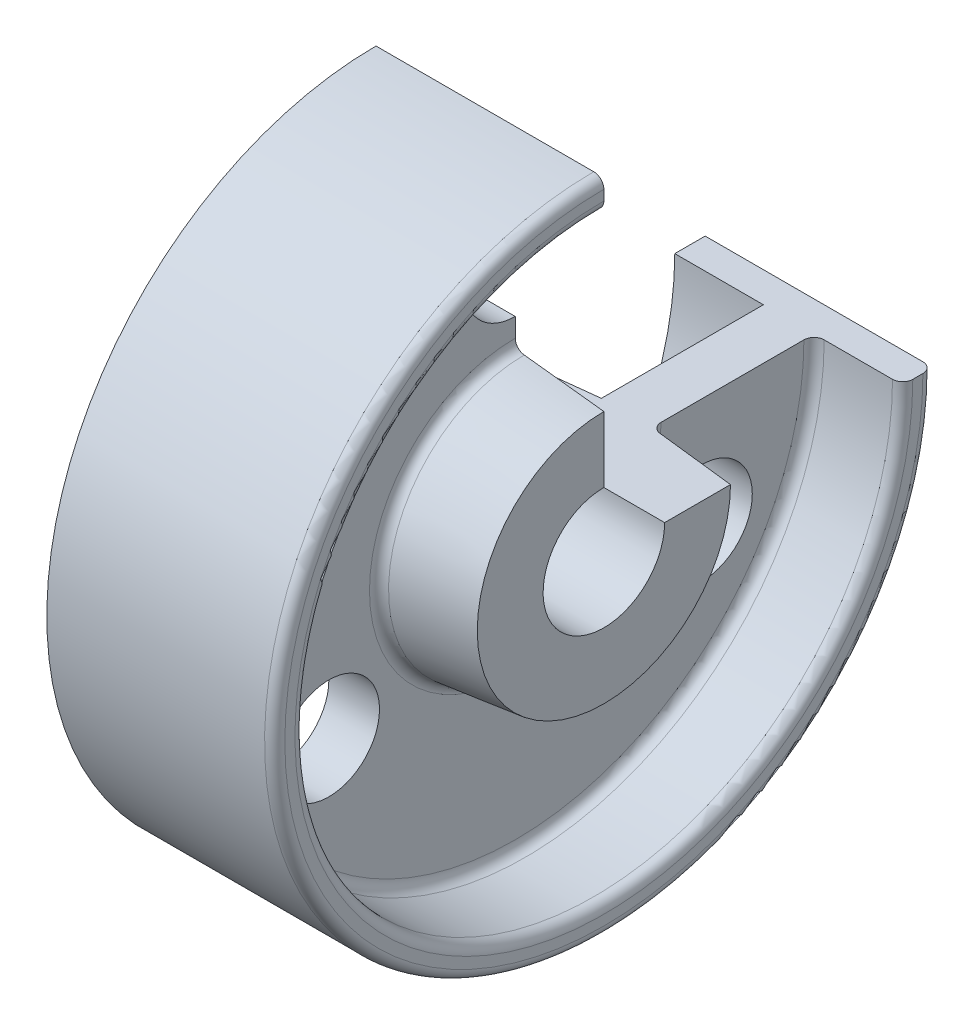
ISO-10303-21;
HEADER;
FILE_DESCRIPTION(('STEP AP214'),'2;1');
FILE_NAME('part.step','',(''),(''),'','','');
FILE_SCHEMA(('AUTOMOTIVE_DESIGN { 1 0 10303 214 1 1 1 1 }'));
ENDSEC;
DATA;
#1=APPLICATION_CONTEXT('core data for automotive mechanical design processes');
#2=APPLICATION_PROTOCOL_DEFINITION('international standard','automotive_design',2000,#1);
#3=PRODUCT_CONTEXT('',#1,'mechanical');
#4=PRODUCT('Part','Part','',(#3));
#5=PRODUCT_RELATED_PRODUCT_CATEGORY('part','',(#4));
#6=PRODUCT_DEFINITION_FORMATION('','',#4);
#7=PRODUCT_DEFINITION_CONTEXT('part definition',#1,'design');
#8=PRODUCT_DEFINITION('design','',#6,#7);
#9=PRODUCT_DEFINITION_SHAPE('','',#8);
#10=(LENGTH_UNIT() NAMED_UNIT(*) SI_UNIT(.MILLI.,.METRE.));
#11=(NAMED_UNIT(*) PLANE_ANGLE_UNIT() SI_UNIT($,.RADIAN.));
#12=(NAMED_UNIT(*) SI_UNIT($,.STERADIAN.) SOLID_ANGLE_UNIT());
#13=UNCERTAINTY_MEASURE_WITH_UNIT(LENGTH_MEASURE(1.E-05),#10,'distance_accuracy_value','');
#14=(GEOMETRIC_REPRESENTATION_CONTEXT(3) GLOBAL_UNCERTAINTY_ASSIGNED_CONTEXT((#13)) GLOBAL_UNIT_ASSIGNED_CONTEXT((#10,
#11,#12)) REPRESENTATION_CONTEXT('',''));
#15=CARTESIAN_POINT('',(0.,0.,0.));
#16=DIRECTION('',(0.,0.,1.));
#17=DIRECTION('',(1.,0.,0.));
#18=AXIS2_PLACEMENT_3D('',#15,#16,#17);
#19=CARTESIAN_POINT('',(5.,0.,0.));
#20=DIRECTION('',(-1.,0.,0.));
#21=DIRECTION('',(0.,0.,1.));
#22=AXIS2_PLACEMENT_3D('',#19,#20,#21);
#23=PLANE('',#22);
#24=CARTESIAN_POINT('',(5.,0.,0.));
#25=DIRECTION('',(-1.,0.,0.));
#26=DIRECTION('',(0.,0.,1.));
#27=AXIS2_PLACEMENT_3D('',#24,#25,#26);
#28=CIRCLE('',#27,57.);
#29=CARTESIAN_POINT('',(5.,57.,0.));
#30=VERTEX_POINT('',#29);
#31=CARTESIAN_POINT('',(5.,0.,-57.));
#32=VERTEX_POINT('',#31);
#33=EDGE_CURVE('E319',#30,#32,#28,.F.);
#34=ORIENTED_EDGE('',*,*,#33,.T.);
#35=DIRECTION('',(0.,0.,1.));
#36=VECTOR('',#35,1.);
#37=CARTESIAN_POINT('',(5.,0.,0.));
#38=LINE('',#37,#36);
#39=CARTESIAN_POINT('',(5.,0.,-28.7844474232924));
#40=VERTEX_POINT('',#39);
#41=EDGE_CURVE('E255',#32,#40,#38,.T.);
#42=ORIENTED_EDGE('',*,*,#41,.T.);
#43=CARTESIAN_POINT('',(5.,0.,0.));
#44=DIRECTION('',(-1.,0.,0.));
#45=DIRECTION('',(0.,0.,1.));
#46=AXIS2_PLACEMENT_3D('',#43,#44,#45);
#47=CIRCLE('',#46,28.7844474232924);
#48=CARTESIAN_POINT('',(5.,28.7844474232924,0.));
#49=VERTEX_POINT('',#48);
#50=EDGE_CURVE('E314',#40,#49,#47,.T.);
#51=ORIENTED_EDGE('',*,*,#50,.T.);
#52=DIRECTION('',(0.,1.,0.));
#53=VECTOR('',#52,1.);
#54=CARTESIAN_POINT('',(5.,0.,0.));
#55=LINE('',#54,#53);
#56=CARTESIAN_POINT('',(5.,32.5,0.));
#57=VERTEX_POINT('',#56);
#58=EDGE_CURVE('E57',#49,#57,#55,.T.);
#59=ORIENTED_EDGE('',*,*,#58,.T.);
#60=CARTESIAN_POINT('',(5.,42.5,0.));
#61=DIRECTION('',(1.,0.,0.));
#62=DIRECTION('',(0.,0.,-1.));
#63=AXIS2_PLACEMENT_3D('',#60,#61,#62);
#64=CIRCLE('',#63,10.);
#65=CARTESIAN_POINT('',(5.,52.5,0.));
#66=VERTEX_POINT('',#65);
#67=EDGE_CURVE('E271',#66,#57,#64,.T.);
#68=ORIENTED_EDGE('',*,*,#67,.F.);
#69=EDGE_CURVE('E221',#66,#30,#55,.T.);
#70=ORIENTED_EDGE('',*,*,#69,.T.);
#71=EDGE_LOOP('',(#34,#42,#51,#59,#68,#70));
#72=FACE_BOUND('',#71,.T.);
#73=CARTESIAN_POINT('',(5.,-21.250000000001,36.806079660838));
#74=DIRECTION('',(1.,0.,0.));
#75=DIRECTION('',(0.,0.,-1.));
#76=AXIS2_PLACEMENT_3D('',#73,#74,#75);
#77=CIRCLE('',#76,10.0000000000015);
#78=CARTESIAN_POINT('',(5.,-21.250000000001,26.8060796608365));
#79=VERTEX_POINT('',#78);
#80=EDGE_CURVE('E280',#79,#79,#77,.T.);
#81=ORIENTED_EDGE('',*,*,#80,.F.);
#82=EDGE_LOOP('',(#81));
#83=FACE_BOUND('',#82,.T.);
#84=CARTESIAN_POINT('',(5.,-21.25,-36.8060796608398));
#85=DIRECTION('',(1.,0.,0.));
#86=DIRECTION('',(0.,0.,-1.));
#87=AXIS2_PLACEMENT_3D('',#84,#85,#86);
#88=CIRCLE('',#87,10.0000000000005);
#89=CARTESIAN_POINT('',(5.,-21.25,-46.8060796608403));
#90=VERTEX_POINT('',#89);
#91=EDGE_CURVE('E275',#90,#90,#88,.T.);
#92=ORIENTED_EDGE('',*,*,#91,.F.);
#93=EDGE_LOOP('',(#92));
#94=FACE_BOUND('',#93,.T.);
#95=ADVANCED_FACE('F41',(#72,#83,#94),#23,.F.);
#96=CARTESIAN_POINT('',(-22.5,0.,0.));
#97=DIRECTION('',(-1.,0.,0.));
#98=DIRECTION('',(0.,0.,1.));
#99=AXIS2_PLACEMENT_3D('',#96,#97,#98);
#100=PLANE('',#99);
#101=DIRECTION('',(0.,0.,-1.));
#102=VECTOR('',#101,1.);
#103=CARTESIAN_POINT('',(-22.5,0.,0.));
#104=LINE('',#103,#102);
#105=CARTESIAN_POINT('',(-22.5,0.,-12.));
#106=VERTEX_POINT('',#105);
#107=CARTESIAN_POINT('',(-22.5,0.,-25.));
#108=VERTEX_POINT('',#107);
#109=EDGE_CURVE('E206',#106,#108,#104,.T.);
#110=ORIENTED_EDGE('',*,*,#109,.T.);
#111=CARTESIAN_POINT('',(-22.5,0.,0.));
#112=DIRECTION('',(-1.,0.,0.));
#113=DIRECTION('',(0.,0.,1.));
#114=AXIS2_PLACEMENT_3D('',#111,#112,#113);
#115=CIRCLE('',#114,25.);
#116=CARTESIAN_POINT('',(-22.5,25.,0.));
#117=VERTEX_POINT('',#116);
#118=EDGE_CURVE('E281',#108,#117,#115,.T.);
#119=ORIENTED_EDGE('',*,*,#118,.T.);
#120=DIRECTION('',(0.,-1.,0.));
#121=VECTOR('',#120,1.);
#122=CARTESIAN_POINT('',(-22.5,77.9926066109058,0.));
#123=LINE('',#122,#121);
#124=CARTESIAN_POINT('',(-22.5,12.,0.));
#125=VERTEX_POINT('',#124);
#126=EDGE_CURVE('E219',#117,#125,#123,.T.);
#127=ORIENTED_EDGE('',*,*,#126,.T.);
#128=CARTESIAN_POINT('',(-22.5,0.,0.));
#129=DIRECTION('',(-1.,0.,0.));
#130=DIRECTION('',(0.,0.,1.));
#131=AXIS2_PLACEMENT_3D('',#128,#129,#130);
#132=CIRCLE('',#131,12.);
#133=EDGE_CURVE('E302',#106,#125,#132,.T.);
#134=ORIENTED_EDGE('',*,*,#133,.F.);
#135=EDGE_LOOP('',(#110,#119,#127,#134));
#136=FACE_BOUND('',#135,.T.);
#137=ADVANCED_FACE('F366',(#136),#100,.T.);
#138=CARTESIAN_POINT('',(-53.0847305724635,0.,0.));
#139=DIRECTION('',(-1.,0.,0.));
#140=DIRECTION('',(0.,0.,1.));
#141=AXIS2_PLACEMENT_3D('',#138,#139,#140);
#142=CYLINDRICAL_SURFACE('',#141,12.);
#143=DIRECTION('',(-1.,0.,0.));
#144=VECTOR('',#143,1.);
#145=CARTESIAN_POINT('',(-53.0847305724635,0.,-12.));
#146=LINE('',#145,#144);
#147=CARTESIAN_POINT('',(22.5,0.,-12.));
#148=VERTEX_POINT('',#147);
#149=EDGE_CURVE('E266',#106,#148,#146,.F.);
#150=ORIENTED_EDGE('',*,*,#149,.F.);
#151=ORIENTED_EDGE('',*,*,#133,.T.);
#152=DIRECTION('',(-1.,0.,0.));
#153=VECTOR('',#152,1.);
#154=CARTESIAN_POINT('',(-53.0847305724635,12.,0.));
#155=LINE('',#154,#153);
#156=CARTESIAN_POINT('',(22.5,12.,0.));
#157=VERTEX_POINT('',#156);
#158=EDGE_CURVE('E246',#157,#125,#155,.T.);
#159=ORIENTED_EDGE('',*,*,#158,.F.);
#160=CARTESIAN_POINT('',(22.5,0.,0.));
#161=DIRECTION('',(-1.,0.,0.));
#162=DIRECTION('',(0.,0.,1.));
#163=AXIS2_PLACEMENT_3D('',#160,#161,#162);
#164=CIRCLE('',#163,12.);
#165=EDGE_CURVE('E301',#148,#157,#164,.T.);
#166=ORIENTED_EDGE('',*,*,#165,.F.);
#167=EDGE_LOOP('',(#150,#151,#159,#166));
#168=FACE_BOUND('',#167,.T.);
#169=ADVANCED_FACE('F367',(#168),#142,.F.);
#170=CARTESIAN_POINT('',(22.5,0.,0.));
#171=DIRECTION('',(-1.,0.,0.));
#172=DIRECTION('',(0.,0.,1.));
#173=AXIS2_PLACEMENT_3D('',#170,#171,#172);
#174=PLANE('',#173);
#175=CARTESIAN_POINT('',(22.5,0.,0.));
#176=DIRECTION('',(-1.,0.,0.));
#177=DIRECTION('',(0.,0.,1.));
#178=AXIS2_PLACEMENT_3D('',#175,#176,#177);
#179=CIRCLE('',#178,25.);
#180=CARTESIAN_POINT('',(22.5,0.,-25.));
#181=VERTEX_POINT('',#180);
#182=CARTESIAN_POINT('',(22.5,25.,0.));
#183=VERTEX_POINT('',#182);
#184=EDGE_CURVE('E296',#181,#183,#179,.T.);
#185=ORIENTED_EDGE('',*,*,#184,.F.);
#186=DIRECTION('',(0.,0.,-1.));
#187=VECTOR('',#186,1.);
#188=CARTESIAN_POINT('',(22.5,0.,0.));
#189=LINE('',#188,#187);
#190=EDGE_CURVE('E211',#148,#181,#189,.T.);
#191=ORIENTED_EDGE('',*,*,#190,.F.);
#192=ORIENTED_EDGE('',*,*,#165,.T.);
#193=DIRECTION('',(0.,-1.,0.));
#194=VECTOR('',#193,1.);
#195=CARTESIAN_POINT('',(22.5,77.9926066109058,0.));
#196=LINE('',#195,#194);
#197=EDGE_CURVE('E185',#183,#157,#196,.T.);
#198=ORIENTED_EDGE('',*,*,#197,.F.);
#199=EDGE_LOOP('',(#185,#191,#192,#198));
#200=FACE_BOUND('',#199,.T.);
#201=ADVANCED_FACE('F373',(#200),#174,.F.);
#202=CARTESIAN_POINT('',(22.5,0.,0.));
#203=DIRECTION('',(-1.,0.,0.));
#204=DIRECTION('',(0.,0.,1.));
#205=AXIS2_PLACEMENT_3D('',#202,#203,#204);
#206=CONICAL_SURFACE('',#205,25.,0.113792007143708);
#207=CARTESIAN_POINT('',(6.77290681767853,0.,0.));
#208=DIRECTION('',(-1.,0.,0.));
#209=DIRECTION('',(0.,0.,1.));
#210=AXIS2_PLACEMENT_3D('',#207,#208,#209);
#211=CIRCLE('',#210,26.7973820779796);
#212=CARTESIAN_POINT('',(6.77290681767853,26.7973820779796,0.));
#213=VERTEX_POINT('',#212);
#214=CARTESIAN_POINT('',(6.77290681767853,0.,-26.7973820779796));
#215=VERTEX_POINT('',#214);
#216=EDGE_CURVE('E192',#213,#215,#211,.F.);
#217=ORIENTED_EDGE('',*,*,#216,.T.);
#218=DIRECTION('',(0.993532672656404,0.,0.113546591160732));
#219=VECTOR('',#218,1.);
#220=CARTESIAN_POINT('',(241.25,0.,0.));
#221=LINE('',#220,#219);
#222=EDGE_CURVE('E259',#215,#181,#221,.T.);
#223=ORIENTED_EDGE('',*,*,#222,.T.);
#224=ORIENTED_EDGE('',*,*,#184,.T.);
#225=DIRECTION('',(-0.993532672656404,0.113546591160732,0.));
#226=VECTOR('',#225,1.);
#227=CARTESIAN_POINT('',(241.25,0.,0.));
#228=LINE('',#227,#226);
#229=EDGE_CURVE('E238',#183,#213,#228,.T.);
#230=ORIENTED_EDGE('',*,*,#229,.T.);
#231=EDGE_LOOP('',(#217,#223,#224,#230));
#232=FACE_BOUND('',#231,.T.);
#233=ADVANCED_FACE('F324',(#232),#206,.T.);
#234=CARTESIAN_POINT('',(-53.0847305724635,0.,0.));
#235=DIRECTION('',(-1.,0.,0.));
#236=DIRECTION('',(0.,0.,1.));
#237=AXIS2_PLACEMENT_3D('',#234,#235,#236);
#238=CYLINDRICAL_SURFACE('',#237,59.);
#239=CARTESIAN_POINT('',(20.5,0.,0.));
#240=DIRECTION('',(-1.,0.,0.));
#241=DIRECTION('',(0.,0.,1.));
#242=AXIS2_PLACEMENT_3D('',#239,#240,#241);
#243=CIRCLE('',#242,59.);
#244=CARTESIAN_POINT('',(20.5,59.,0.));
#245=VERTEX_POINT('',#244);
#246=CARTESIAN_POINT('',(20.5,0.,-59.));
#247=VERTEX_POINT('',#246);
#248=EDGE_CURVE('E186',#245,#247,#243,.F.);
#249=ORIENTED_EDGE('',*,*,#248,.T.);
#250=DIRECTION('',(-1.,0.,0.));
#251=VECTOR('',#250,1.);
#252=CARTESIAN_POINT('',(-53.0847305724635,0.,-59.));
#253=LINE('',#252,#251);
#254=CARTESIAN_POINT('',(7.,0.,-59.));
#255=VERTEX_POINT('',#254);
#256=EDGE_CURVE('E214',#247,#255,#253,.T.);
#257=ORIENTED_EDGE('',*,*,#256,.T.);
#258=CARTESIAN_POINT('',(7.,0.,0.));
#259=DIRECTION('',(-1.,0.,0.));
#260=DIRECTION('',(0.,0.,1.));
#261=AXIS2_PLACEMENT_3D('',#258,#259,#260);
#262=CIRCLE('',#261,59.);
#263=CARTESIAN_POINT('',(7.,59.,0.));
#264=VERTEX_POINT('',#263);
#265=EDGE_CURVE('E207',#255,#264,#262,.T.);
#266=ORIENTED_EDGE('',*,*,#265,.T.);
#267=DIRECTION('',(-1.,0.,0.));
#268=VECTOR('',#267,1.);
#269=CARTESIAN_POINT('',(-53.0847305724635,59.,0.));
#270=LINE('',#269,#268);
#271=EDGE_CURVE('E196',#264,#245,#270,.F.);
#272=ORIENTED_EDGE('',*,*,#271,.T.);
#273=EDGE_LOOP('',(#249,#257,#266,#272));
#274=FACE_BOUND('',#273,.T.);
#275=ADVANCED_FACE('F202',(#274),#238,.F.);
#276=CARTESIAN_POINT('',(22.5,0.,0.));
#277=DIRECTION('',(-1.,0.,0.));
#278=DIRECTION('',(0.,0.,1.));
#279=AXIS2_PLACEMENT_3D('',#276,#277,#278);
#280=PLANE('',#279);
#281=CARTESIAN_POINT('',(22.5,0.,0.));
#282=DIRECTION('',(-1.,0.,0.));
#283=DIRECTION('',(0.,0.,1.));
#284=AXIS2_PLACEMENT_3D('',#281,#282,#283);
#285=CIRCLE('',#284,63.);
#286=CARTESIAN_POINT('',(22.5,63.,0.));
#287=VERTEX_POINT('',#286);
#288=CARTESIAN_POINT('',(22.5,0.,-63.));
#289=VERTEX_POINT('',#288);
#290=EDGE_CURVE('E178',#287,#289,#285,.F.);
#291=ORIENTED_EDGE('',*,*,#290,.T.);
#292=CARTESIAN_POINT('',(22.5,0.,-61.));
#293=VERTEX_POINT('',#292);
#294=EDGE_CURVE('E181',#293,#289,#189,.T.);
#295=ORIENTED_EDGE('',*,*,#294,.F.);
#296=CARTESIAN_POINT('',(22.5,0.,0.));
#297=DIRECTION('',(-1.,0.,0.));
#298=DIRECTION('',(0.,0.,1.));
#299=AXIS2_PLACEMENT_3D('',#296,#297,#298);
#300=CIRCLE('',#299,61.);
#301=CARTESIAN_POINT('',(22.5,61.,0.));
#302=VERTEX_POINT('',#301);
#303=EDGE_CURVE('E179',#293,#302,#300,.T.);
#304=ORIENTED_EDGE('',*,*,#303,.T.);
#305=EDGE_CURVE('E61',#287,#302,#196,.T.);
#306=ORIENTED_EDGE('',*,*,#305,.F.);
#307=EDGE_LOOP('',(#291,#295,#304,#306));
#308=FACE_BOUND('',#307,.T.);
#309=ADVANCED_FACE('F176',(#308),#280,.F.);
#310=CARTESIAN_POINT('',(-53.0847305724635,0.,0.));
#311=DIRECTION('',(-1.,0.,0.));
#312=DIRECTION('',(0.,0.,1.));
#313=AXIS2_PLACEMENT_3D('',#310,#311,#312);
#314=CYLINDRICAL_SURFACE('',#313,65.);
#315=DIRECTION('',(-1.,0.,0.));
#316=VECTOR('',#315,1.);
#317=CARTESIAN_POINT('',(-53.0847305724635,0.,-65.));
#318=LINE('',#317,#316);
#319=CARTESIAN_POINT('',(20.5,0.,-65.));
#320=VERTEX_POINT('',#319);
#321=CARTESIAN_POINT('',(-22.5,0.,-65.));
#322=VERTEX_POINT('',#321);
#323=EDGE_CURVE('E261',#320,#322,#318,.T.);
#324=ORIENTED_EDGE('',*,*,#323,.F.);
#325=CARTESIAN_POINT('',(20.5,0.,0.));
#326=DIRECTION('',(-1.,0.,0.));
#327=DIRECTION('',(0.,0.,1.));
#328=AXIS2_PLACEMENT_3D('',#325,#326,#327);
#329=CIRCLE('',#328,65.);
#330=CARTESIAN_POINT('',(20.5,65.,0.));
#331=VERTEX_POINT('',#330);
#332=EDGE_CURVE('E190',#320,#331,#329,.T.);
#333=ORIENTED_EDGE('',*,*,#332,.T.);
#334=DIRECTION('',(-1.,0.,0.));
#335=VECTOR('',#334,1.);
#336=CARTESIAN_POINT('',(-53.0847305724635,65.,0.));
#337=LINE('',#336,#335);
#338=CARTESIAN_POINT('',(-22.5,65.,0.));
#339=VERTEX_POINT('',#338);
#340=EDGE_CURVE('E168',#339,#331,#337,.F.);
#341=ORIENTED_EDGE('',*,*,#340,.F.);
#342=CARTESIAN_POINT('',(-22.5,0.,0.));
#343=DIRECTION('',(-1.,0.,0.));
#344=DIRECTION('',(0.,0.,1.));
#345=AXIS2_PLACEMENT_3D('',#342,#343,#344);
#346=CIRCLE('',#345,65.);
#347=EDGE_CURVE('E294',#322,#339,#346,.T.);
#348=ORIENTED_EDGE('',*,*,#347,.F.);
#349=EDGE_LOOP('',(#324,#333,#341,#348));
#350=FACE_BOUND('',#349,.T.);
#351=ADVANCED_FACE('F358',(#350),#314,.T.);
#352=CARTESIAN_POINT('',(-22.5,0.,0.));
#353=DIRECTION('',(-1.,0.,0.));
#354=DIRECTION('',(0.,0.,1.));
#355=AXIS2_PLACEMENT_3D('',#352,#353,#354);
#356=PLANE('',#355);
#357=CARTESIAN_POINT('',(-22.5,0.,-59.));
#358=VERTEX_POINT('',#357);
#359=EDGE_CURVE('E223',#358,#322,#104,.T.);
#360=ORIENTED_EDGE('',*,*,#359,.T.);
#361=ORIENTED_EDGE('',*,*,#347,.T.);
#362=CARTESIAN_POINT('',(-22.5,59.,0.));
#363=VERTEX_POINT('',#362);
#364=EDGE_CURVE('E217',#339,#363,#123,.T.);
#365=ORIENTED_EDGE('',*,*,#364,.T.);
#366=CARTESIAN_POINT('',(-22.5,0.,0.));
#367=DIRECTION('',(-1.,0.,0.));
#368=DIRECTION('',(0.,0.,1.));
#369=AXIS2_PLACEMENT_3D('',#366,#367,#368);
#370=CIRCLE('',#369,59.);
#371=EDGE_CURVE('E292',#358,#363,#370,.T.);
#372=ORIENTED_EDGE('',*,*,#371,.F.);
#373=EDGE_LOOP('',(#360,#361,#365,#372));
#374=FACE_BOUND('',#373,.T.);
#375=ADVANCED_FACE('F354',(#374),#356,.T.);
#376=CARTESIAN_POINT('',(-53.0847305724635,0.,0.));
#377=DIRECTION('',(-1.,0.,0.));
#378=DIRECTION('',(0.,0.,1.));
#379=AXIS2_PLACEMENT_3D('',#376,#377,#378);
#380=CYLINDRICAL_SURFACE('',#379,59.);
#381=DIRECTION('',(-1.,0.,0.));
#382=VECTOR('',#381,1.);
#383=CARTESIAN_POINT('',(-53.0847305724635,0.,-59.));
#384=LINE('',#383,#382);
#385=CARTESIAN_POINT('',(-5.,0.,-59.));
#386=VERTEX_POINT('',#385);
#387=EDGE_CURVE('E267',#358,#386,#384,.F.);
#388=ORIENTED_EDGE('',*,*,#387,.F.);
#389=ORIENTED_EDGE('',*,*,#371,.T.);
#390=DIRECTION('',(-1.,0.,0.));
#391=VECTOR('',#390,1.);
#392=CARTESIAN_POINT('',(-53.0847305724635,59.,0.));
#393=LINE('',#392,#391);
#394=CARTESIAN_POINT('',(-5.,59.,0.));
#395=VERTEX_POINT('',#394);
#396=EDGE_CURVE('E171',#395,#363,#393,.T.);
#397=ORIENTED_EDGE('',*,*,#396,.F.);
#398=CARTESIAN_POINT('',(-5.,0.,0.));
#399=DIRECTION('',(-1.,0.,0.));
#400=DIRECTION('',(0.,0.,1.));
#401=AXIS2_PLACEMENT_3D('',#398,#399,#400);
#402=CIRCLE('',#401,59.);
#403=EDGE_CURVE('E290',#386,#395,#402,.T.);
#404=ORIENTED_EDGE('',*,*,#403,.F.);
#405=EDGE_LOOP('',(#388,#389,#397,#404));
#406=FACE_BOUND('',#405,.T.);
#407=ADVANCED_FACE('F348',(#406),#380,.F.);
#408=CARTESIAN_POINT('',(-5.,0.,0.));
#409=DIRECTION('',(-1.,0.,0.));
#410=DIRECTION('',(0.,0.,1.));
#411=AXIS2_PLACEMENT_3D('',#408,#409,#410);
#412=PLANE('',#411);
#413=DIRECTION('',(0.,0.,1.));
#414=VECTOR('',#413,1.);
#415=CARTESIAN_POINT('',(-5.,0.,0.));
#416=LINE('',#415,#414);
#417=CARTESIAN_POINT('',(-5.,0.,-27.));
#418=VERTEX_POINT('',#417);
#419=EDGE_CURVE('E268',#386,#418,#416,.T.);
#420=ORIENTED_EDGE('',*,*,#419,.F.);
#421=ORIENTED_EDGE('',*,*,#403,.T.);
#422=DIRECTION('',(0.,1.,0.));
#423=VECTOR('',#422,1.);
#424=CARTESIAN_POINT('',(-5.,0.,0.));
#425=LINE('',#424,#423);
#426=CARTESIAN_POINT('',(-5.,52.5,0.));
#427=VERTEX_POINT('',#426);
#428=EDGE_CURVE('E233',#427,#395,#425,.T.);
#429=ORIENTED_EDGE('',*,*,#428,.F.);
#430=CARTESIAN_POINT('',(-5.,42.5,0.));
#431=DIRECTION('',(-1.,0.,0.));
#432=DIRECTION('',(0.,0.,1.));
#433=AXIS2_PLACEMENT_3D('',#430,#431,#432);
#434=CIRCLE('',#433,10.);
#435=CARTESIAN_POINT('',(-5.,32.5,0.));
#436=VERTEX_POINT('',#435);
#437=EDGE_CURVE('E288',#436,#427,#434,.T.);
#438=ORIENTED_EDGE('',*,*,#437,.F.);
#439=CARTESIAN_POINT('',(-5.,27.,0.));
#440=VERTEX_POINT('',#439);
#441=EDGE_CURVE('E231',#440,#436,#425,.T.);
#442=ORIENTED_EDGE('',*,*,#441,.F.);
#443=CARTESIAN_POINT('',(-5.,0.,0.));
#444=DIRECTION('',(-1.,0.,0.));
#445=DIRECTION('',(0.,0.,1.));
#446=AXIS2_PLACEMENT_3D('',#443,#444,#445);
#447=CIRCLE('',#446,27.);
#448=EDGE_CURVE('E282',#418,#440,#447,.T.);
#449=ORIENTED_EDGE('',*,*,#448,.F.);
#450=EDGE_LOOP('',(#420,#421,#429,#438,#442,#449));
#451=FACE_BOUND('',#450,.T.);
#452=CARTESIAN_POINT('',(-5.,-21.250000000001,36.806079660838));
#453=DIRECTION('',(-1.,0.,0.));
#454=DIRECTION('',(0.,0.,1.));
#455=AXIS2_PLACEMENT_3D('',#452,#453,#454);
#456=CIRCLE('',#455,10.0000000000015);
#457=CARTESIAN_POINT('',(-5.,-21.250000000001,46.8060796608396));
#458=VERTEX_POINT('',#457);
#459=EDGE_CURVE('E307',#458,#458,#456,.T.);
#460=ORIENTED_EDGE('',*,*,#459,.F.);
#461=EDGE_LOOP('',(#460));
#462=FACE_BOUND('',#461,.T.);
#463=CARTESIAN_POINT('',(-5.,-21.25,-36.8060796608398));
#464=DIRECTION('',(-1.,0.,0.));
#465=DIRECTION('',(0.,0.,1.));
#466=AXIS2_PLACEMENT_3D('',#463,#464,#465);
#467=CIRCLE('',#466,10.0000000000005);
#468=CARTESIAN_POINT('',(-5.,-21.25,-26.8060796608393));
#469=VERTEX_POINT('',#468);
#470=EDGE_CURVE('E277',#469,#469,#467,.T.);
#471=ORIENTED_EDGE('',*,*,#470,.F.);
#472=EDGE_LOOP('',(#471));
#473=FACE_BOUND('',#472,.T.);
#474=ADVANCED_FACE('F342',(#451,#462,#473),#412,.T.);
#475=CARTESIAN_POINT('',(-22.5,0.,0.));
#476=DIRECTION('',(1.,0.,0.));
#477=DIRECTION('',(0.,0.,-1.));
#478=AXIS2_PLACEMENT_3D('',#475,#476,#477);
#479=CONICAL_SURFACE('',#478,25.,0.113792007143708);
#480=DIRECTION('',(0.993532672656404,0.,-0.113546591160732));
#481=VECTOR('',#480,1.);
#482=CARTESIAN_POINT('',(-241.250000000001,0.,0.));
#483=LINE('',#482,#481);
#484=EDGE_CURVE('E263',#418,#108,#483,.F.);
#485=ORIENTED_EDGE('',*,*,#484,.F.);
#486=ORIENTED_EDGE('',*,*,#448,.T.);
#487=DIRECTION('',(-0.993532672656404,-0.113546591160732,0.));
#488=VECTOR('',#487,1.);
#489=CARTESIAN_POINT('',(-241.250000000001,0.,0.));
#490=LINE('',#489,#488);
#491=EDGE_CURVE('E242',#117,#440,#490,.F.);
#492=ORIENTED_EDGE('',*,*,#491,.F.);
#493=ORIENTED_EDGE('',*,*,#118,.F.);
#494=EDGE_LOOP('',(#485,#486,#492,#493));
#495=FACE_BOUND('',#494,.T.);
#496=ADVANCED_FACE('F359',(#495),#479,.T.);
#497=CARTESIAN_POINT('',(-22.5,-21.25,-36.8060796608398));
#498=DIRECTION('',(1.,0.,0.));
#499=DIRECTION('',(0.,0.,-1.));
#500=AXIS2_PLACEMENT_3D('',#497,#498,#499);
#501=CYLINDRICAL_SURFACE('',#500,10.0000000000005);
#502=ORIENTED_EDGE('',*,*,#470,.T.);
#503=EDGE_LOOP('',(#502));
#504=FACE_BOUND('',#503,.T.);
#505=ORIENTED_EDGE('',*,*,#91,.T.);
#506=EDGE_LOOP('',(#505));
#507=FACE_BOUND('',#506,.T.);
#508=ADVANCED_FACE('F451',(#504,#507),#501,.F.);
#509=CARTESIAN_POINT('',(-22.5,-21.250000000001,36.806079660838));
#510=DIRECTION('',(1.,0.,0.));
#511=DIRECTION('',(0.,0.,-1.));
#512=AXIS2_PLACEMENT_3D('',#509,#510,#511);
#513=CYLINDRICAL_SURFACE('',#512,10.0000000000015);
#514=ORIENTED_EDGE('',*,*,#459,.T.);
#515=EDGE_LOOP('',(#514));
#516=FACE_BOUND('',#515,.T.);
#517=ORIENTED_EDGE('',*,*,#80,.T.);
#518=EDGE_LOOP('',(#517));
#519=FACE_BOUND('',#518,.T.);
#520=ADVANCED_FACE('F449',(#516,#519),#513,.F.);
#521=CARTESIAN_POINT('',(-22.5,42.5,0.));
#522=DIRECTION('',(1.,0.,0.));
#523=DIRECTION('',(0.,0.,-1.));
#524=AXIS2_PLACEMENT_3D('',#521,#522,#523);
#525=CYLINDRICAL_SURFACE('',#524,10.);
#526=ORIENTED_EDGE('',*,*,#67,.T.);
#527=DIRECTION('',(1.,0.,0.));
#528=VECTOR('',#527,1.);
#529=CARTESIAN_POINT('',(-22.5,32.5,0.));
#530=LINE('',#529,#528);
#531=EDGE_CURVE('E241',#57,#436,#530,.F.);
#532=ORIENTED_EDGE('',*,*,#531,.T.);
#533=ORIENTED_EDGE('',*,*,#437,.T.);
#534=DIRECTION('',(1.,0.,0.));
#535=VECTOR('',#534,1.);
#536=CARTESIAN_POINT('',(-22.5,52.5,0.));
#537=LINE('',#536,#535);
#538=EDGE_CURVE('E226',#427,#66,#537,.T.);
#539=ORIENTED_EDGE('',*,*,#538,.T.);
#540=EDGE_LOOP('',(#526,#532,#533,#539));
#541=FACE_BOUND('',#540,.T.);
#542=ADVANCED_FACE('F337',(#541),#525,.F.);
#543=CARTESIAN_POINT('',(7.,0.,0.));
#544=DIRECTION('',(-1.,0.,0.));
#545=DIRECTION('',(0.,0.,1.));
#546=AXIS2_PLACEMENT_3D('',#543,#544,#545);
#547=TOROIDAL_SURFACE('',#546,57.,2.);
#548=ORIENTED_EDGE('',*,*,#265,.F.);
#549=CARTESIAN_POINT('',(7.,0.,-57.));
#550=DIRECTION('',(0.,-1.,0.));
#551=DIRECTION('',(0.,0.,-1.));
#552=AXIS2_PLACEMENT_3D('',#549,#550,#551);
#553=CIRCLE('',#552,2.);
#554=EDGE_CURVE('E248',#255,#32,#553,.F.);
#555=ORIENTED_EDGE('',*,*,#554,.T.);
#556=ORIENTED_EDGE('',*,*,#33,.F.);
#557=CARTESIAN_POINT('',(7.,57.,0.));
#558=DIRECTION('',(0.,0.,1.));
#559=DIRECTION('',(1.,0.,0.));
#560=AXIS2_PLACEMENT_3D('',#557,#558,#559);
#561=CIRCLE('',#560,2.);
#562=EDGE_CURVE('E210',#30,#264,#561,.F.);
#563=ORIENTED_EDGE('',*,*,#562,.T.);
#564=EDGE_LOOP('',(#548,#555,#556,#563));
#565=FACE_BOUND('',#564,.T.);
#566=ADVANCED_FACE('F332',(#565),#547,.F.);
#567=CARTESIAN_POINT('',(7.,0.,0.));
#568=DIRECTION('',(-1.,0.,0.));
#569=DIRECTION('',(0.,0.,1.));
#570=AXIS2_PLACEMENT_3D('',#567,#568,#569);
#571=TOROIDAL_SURFACE('',#570,28.7844474232924,2.);
#572=ORIENTED_EDGE('',*,*,#50,.F.);
#573=CARTESIAN_POINT('',(7.,0.,-28.7844474232924));
#574=DIRECTION('',(0.,-1.,0.));
#575=DIRECTION('',(0.,0.,-1.));
#576=AXIS2_PLACEMENT_3D('',#573,#574,#575);
#577=CIRCLE('',#576,2.);
#578=EDGE_CURVE('E253',#40,#215,#577,.F.);
#579=ORIENTED_EDGE('',*,*,#578,.T.);
#580=ORIENTED_EDGE('',*,*,#216,.F.);
#581=CARTESIAN_POINT('',(7.,28.7844474232924,0.));
#582=DIRECTION('',(0.,0.,1.));
#583=DIRECTION('',(1.,0.,0.));
#584=AXIS2_PLACEMENT_3D('',#581,#582,#583);
#585=CIRCLE('',#584,2.);
#586=EDGE_CURVE('E236',#213,#49,#585,.F.);
#587=ORIENTED_EDGE('',*,*,#586,.T.);
#588=EDGE_LOOP('',(#572,#579,#580,#587));
#589=FACE_BOUND('',#588,.T.);
#590=ADVANCED_FACE('F326',(#589),#571,.F.);
#591=CARTESIAN_POINT('',(20.5,0.,0.));
#592=DIRECTION('',(-1.,0.,0.));
#593=DIRECTION('',(0.,0.,1.));
#594=AXIS2_PLACEMENT_3D('',#591,#592,#593);
#595=TOROIDAL_SURFACE('',#594,63.,2.);
#596=CARTESIAN_POINT('',(20.5,0.,-63.));
#597=DIRECTION('',(0.,-1.,0.));
#598=DIRECTION('',(0.,0.,-1.));
#599=AXIS2_PLACEMENT_3D('',#596,#597,#598);
#600=CIRCLE('',#599,2.);
#601=EDGE_CURVE('E187',#289,#320,#600,.F.);
#602=ORIENTED_EDGE('',*,*,#601,.F.);
#603=ORIENTED_EDGE('',*,*,#290,.F.);
#604=CARTESIAN_POINT('',(20.5,63.,0.));
#605=DIRECTION('',(0.,0.,1.));
#606=DIRECTION('',(1.,0.,0.));
#607=AXIS2_PLACEMENT_3D('',#604,#605,#606);
#608=CIRCLE('',#607,2.);
#609=EDGE_CURVE('E161',#331,#287,#608,.F.);
#610=ORIENTED_EDGE('',*,*,#609,.F.);
#611=ORIENTED_EDGE('',*,*,#332,.F.);
#612=EDGE_LOOP('',(#602,#603,#610,#611));
#613=FACE_BOUND('',#612,.T.);
#614=ADVANCED_FACE('F184',(#613),#595,.T.);
#615=CARTESIAN_POINT('',(20.5,0.,0.));
#616=DIRECTION('',(-1.,0.,0.));
#617=DIRECTION('',(0.,0.,1.));
#618=AXIS2_PLACEMENT_3D('',#615,#616,#617);
#619=TOROIDAL_SURFACE('',#618,61.,2.);
#620=CARTESIAN_POINT('',(20.5,0.,-61.));
#621=DIRECTION('',(0.,-1.,0.));
#622=DIRECTION('',(0.,0.,-1.));
#623=AXIS2_PLACEMENT_3D('',#620,#621,#622);
#624=CIRCLE('',#623,2.);
#625=EDGE_CURVE('E11',#247,#293,#624,.F.);
#626=ORIENTED_EDGE('',*,*,#625,.F.);
#627=ORIENTED_EDGE('',*,*,#248,.F.);
#628=CARTESIAN_POINT('',(20.5,61.,0.));
#629=DIRECTION('',(0.,0.,1.));
#630=DIRECTION('',(1.,0.,0.));
#631=AXIS2_PLACEMENT_3D('',#628,#629,#630);
#632=CIRCLE('',#631,2.);
#633=EDGE_CURVE('E47',#302,#245,#632,.F.);
#634=ORIENTED_EDGE('',*,*,#633,.F.);
#635=ORIENTED_EDGE('',*,*,#303,.F.);
#636=EDGE_LOOP('',(#626,#627,#634,#635));
#637=FACE_BOUND('',#636,.T.);
#638=ADVANCED_FACE('F43',(#637),#619,.T.);
#639=CARTESIAN_POINT('',(-22.5,77.9926066109058,0.));
#640=DIRECTION('',(0.,0.,1.));
#641=DIRECTION('',(1.,0.,0.));
#642=AXIS2_PLACEMENT_3D('',#639,#640,#641);
#643=PLANE('',#642);
#644=ORIENTED_EDGE('',*,*,#340,.T.);
#645=ORIENTED_EDGE('',*,*,#609,.T.);
#646=ORIENTED_EDGE('',*,*,#305,.T.);
#647=ORIENTED_EDGE('',*,*,#633,.T.);
#648=ORIENTED_EDGE('',*,*,#271,.F.);
#649=ORIENTED_EDGE('',*,*,#562,.F.);
#650=ORIENTED_EDGE('',*,*,#69,.F.);
#651=ORIENTED_EDGE('',*,*,#538,.F.);
#652=ORIENTED_EDGE('',*,*,#428,.T.);
#653=ORIENTED_EDGE('',*,*,#396,.T.);
#654=ORIENTED_EDGE('',*,*,#364,.F.);
#655=EDGE_LOOP('',(#644,#645,#646,#647,#648,#649,#650,#651,#652,#653,#654));
#656=FACE_BOUND('',#655,.T.);
#657=ADVANCED_FACE('F165',(#656),#643,.F.);
#658=CARTESIAN_POINT('',(-22.5,0.,0.));
#659=DIRECTION('',(0.,-1.,0.));
#660=DIRECTION('',(0.,0.,-1.));
#661=AXIS2_PLACEMENT_3D('',#658,#659,#660);
#662=PLANE('',#661);
#663=ORIENTED_EDGE('',*,*,#149,.T.);
#664=ORIENTED_EDGE('',*,*,#190,.T.);
#665=ORIENTED_EDGE('',*,*,#222,.F.);
#666=ORIENTED_EDGE('',*,*,#578,.F.);
#667=ORIENTED_EDGE('',*,*,#41,.F.);
#668=ORIENTED_EDGE('',*,*,#554,.F.);
#669=ORIENTED_EDGE('',*,*,#256,.F.);
#670=ORIENTED_EDGE('',*,*,#625,.T.);
#671=ORIENTED_EDGE('',*,*,#294,.T.);
#672=ORIENTED_EDGE('',*,*,#601,.T.);
#673=ORIENTED_EDGE('',*,*,#323,.T.);
#674=ORIENTED_EDGE('',*,*,#359,.F.);
#675=ORIENTED_EDGE('',*,*,#387,.T.);
#676=ORIENTED_EDGE('',*,*,#419,.T.);
#677=ORIENTED_EDGE('',*,*,#484,.T.);
#678=ORIENTED_EDGE('',*,*,#109,.F.);
#679=EDGE_LOOP('',(#663,#664,#665,#666,#667,#668,#669,#670,#671,#672,#673,#674,#675,#676,#677,#678));
#680=FACE_BOUND('',#679,.T.);
#681=ADVANCED_FACE('F215',(#680),#662,.F.);
#682=ORIENTED_EDGE('',*,*,#158,.T.);
#683=ORIENTED_EDGE('',*,*,#126,.F.);
#684=ORIENTED_EDGE('',*,*,#491,.T.);
#685=ORIENTED_EDGE('',*,*,#441,.T.);
#686=ORIENTED_EDGE('',*,*,#531,.F.);
#687=ORIENTED_EDGE('',*,*,#58,.F.);
#688=ORIENTED_EDGE('',*,*,#586,.F.);
#689=ORIENTED_EDGE('',*,*,#229,.F.);
#690=ORIENTED_EDGE('',*,*,#197,.T.);
#691=EDGE_LOOP('',(#682,#683,#684,#685,#686,#687,#688,#689,#690));
#692=FACE_BOUND('',#691,.T.);
#693=ADVANCED_FACE('F374',(#692),#643,.F.);
#694=CLOSED_SHELL('',(#95,#137,#169,#201,#233,#275,#309,#351,#375,#407,#474,#496,#508,#520,#542,
#566,#590,#614,#638,#657,#681,#693));
#695=MANIFOLD_SOLID_BREP('B2',#694);
#696=ADVANCED_BREP_SHAPE_REPRESENTATION('',(#18,#695),#14);
#697=SHAPE_DEFINITION_REPRESENTATION(#9,#696);
ENDSEC;
END-ISO-10303-21;
